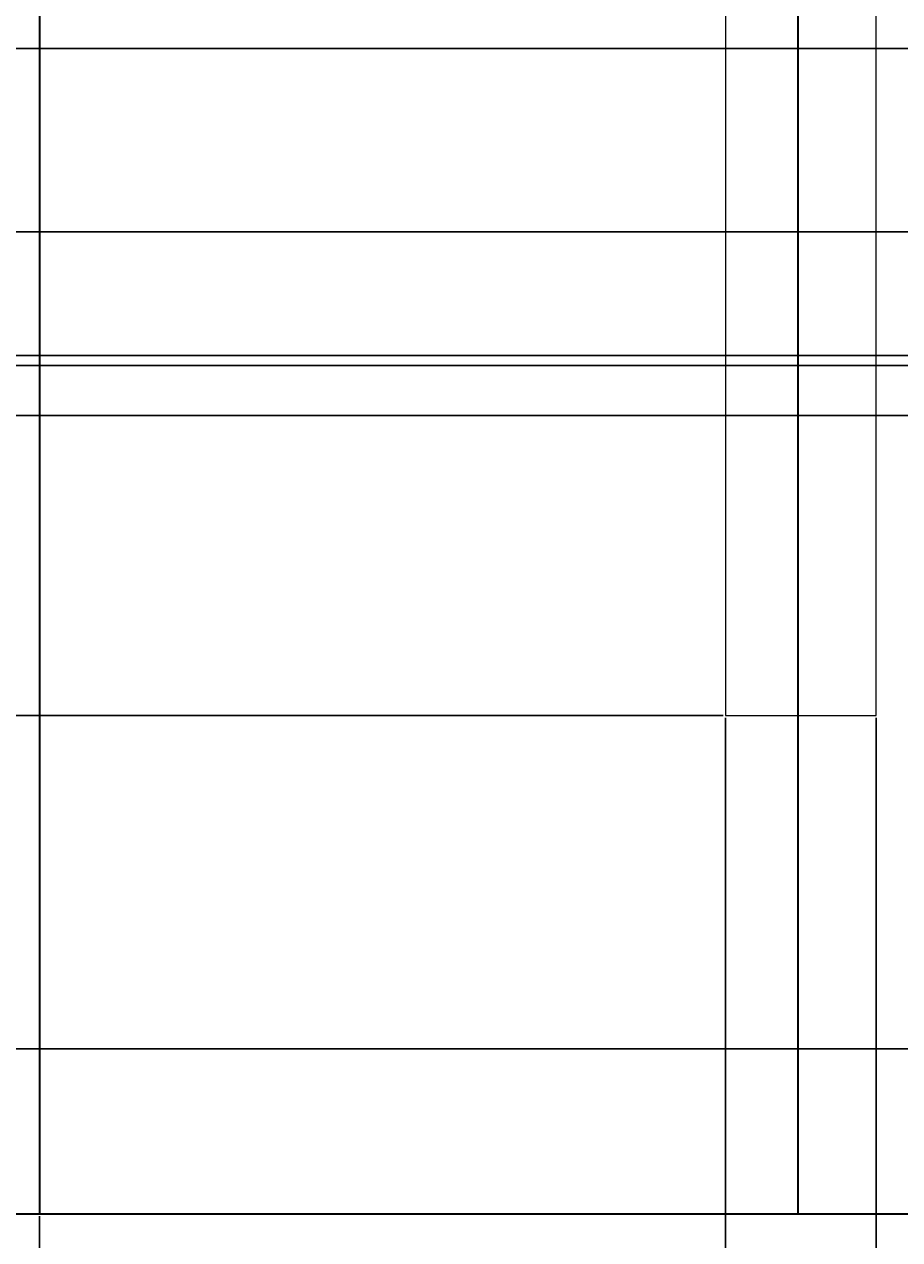
# Model space of a CAD drawing. Units: inches. Extents: x 27 to 200, y -50 to 102.
# Tile 3 of 26: x 44 to 67, y -17 to 15. Entities that reach past the tile are written whole.
import ezdxf

# ---------------------------------------------------------------- set-up
doc = ezdxf.new("R2010")
doc.units = ezdxf.units.IN
doc.header["$MEASUREMENT"] = 0
for name, color, linetype, lineweight in [('A-ANNO-DIMS', 2, 'Continuous', 18), ('A-ELEV', 7, 'Continuous', 35), ('A-EQPM', 9, 'Continuous', 18)]:
    doc.layers.add(name, color=color, linetype=linetype, lineweight=lineweight)
doc.styles.get("Standard").update_dxf_attribs({"font": 'arial.ttf'})
doc.dimstyles.get("Standard").update_dxf_attribs({"dimtxt": 0.18, "dimasz": 0.18, "dimexe": 0.18, "dimexo": 0.0625, "dimgap": 0.09, "dimtad": 0, "dimtih": 1, "dimtoh": 1, "dimdec": 4, "dimzin": 0, "dimdsep": 46, "dimtxsty": 'Standard', "dimcen": 0.09, "dimadec": 0, "dimazin": 0, "dimtfac": 1, "dimtdec": 4, "dimtofl": 0, "dimtmove": 0, "dimatfit": 3, "dimfxl": 1, "dimtolj": 1, "dimtzin": 0, "dimarcsym": 0})

# ---------------------------------------------------------------- blocks, each defined once
blk = doc.blocks.new('*D23')
at = {"layer": 'A-ANNO-DIMS', "color": 0, "lineweight": -2, "transparency": 16777216}
for p, q in [((35.417, -16.832), (35.417, -25.149)), ((191.417, -16.832), (191.417, -25.149)), ((35.597, -24.969), (113.137, -24.969)), ((191.237, -24.969), (113.697, -24.969))]:
    blk.add_line(p, q, dxfattribs=at)
at = {"layer": 'A-ANNO-DIMS', "color": 0, "transparency": 16777216}
for points in [[(35.597, -24.939), (35.597, -24.999), (35.417, -24.969)], [(191.237, -24.939), (191.237, -24.999), (191.417, -24.969)]]:
    blk.add_solid(points, dxfattribs=at)
at = {"layer": 'Defpoints', "color": 0, "transparency": 16777216}
for p in [(35.417, -16.769), (191.417, -16.769), (191.417, -24.969)]:
    blk.add_point(p, dxfattribs=at)
at = {"layer": 'A-ANNO-DIMS', "color": 0, "transparency": 16777216, "insert": (113.417, -24.969), "char_height": 0.18, "attachment_point": 5}
blk.add_mtext('\\A1;156', dxfattribs=at)
blk = doc.blocks.new('*D41')
at = {"layer": 'A-ANNO-DIMS', "color": 0, "lineweight": -2, "transparency": 16777216}
for p, q in [((62.505, -3.679), (62.505, -25.149)), ((44.417, -16.832), (44.417, -25.149)), ((44.597, -24.969), (53.076, -24.969)), ((62.325, -24.969), (53.847, -24.969))]:
    blk.add_line(p, q, dxfattribs=at)
at = {"layer": 'A-ANNO-DIMS', "color": 0, "transparency": 16777216}
for points in [[(44.597, -24.939), (44.597, -24.999), (44.417, -24.969)], [(62.325, -24.939), (62.325, -24.999), (62.505, -24.969)]]:
    blk.add_solid(points, dxfattribs=at)
at = {"layer": 'Defpoints', "color": 0, "transparency": 16777216}
for p in [(62.505, -3.617), (44.417, -16.769), (62.505, -24.969)]:
    blk.add_point(p, dxfattribs=at)
at = {"layer": 'A-ANNO-DIMS', "color": 0, "transparency": 16777216, "insert": (53.461, -24.969), "char_height": 0.18, "attachment_point": 5}
blk.add_mtext('\\A1;18.09', dxfattribs=at)
blk = doc.blocks.new('*D42')
at = {"layer": 'A-ANNO-DIMS', "color": 0, "lineweight": -2, "transparency": 16777216}
for p, q in [((62.505, -3.679), (62.505, -25.149)), ((66.479, -3.679), (66.479, -25.149)), ((62.685, -24.969), (64.098, -24.969)), ((66.299, -24.969), (64.886, -24.969))]:
    blk.add_line(p, q, dxfattribs=at)
at = {"layer": 'A-ANNO-DIMS', "color": 0, "transparency": 16777216}
for points in [[(62.685, -24.939), (62.685, -24.999), (62.505, -24.969)], [(66.299, -24.939), (66.299, -24.999), (66.479, -24.969)]]:
    blk.add_solid(points, dxfattribs=at)
at = {"layer": 'Defpoints', "color": 0, "transparency": 16777216}
for p in [(62.505, -3.617), (66.479, -3.617), (66.479, -24.969)]:
    blk.add_point(p, dxfattribs=at)
at = {"layer": 'A-ANNO-DIMS', "color": 0, "transparency": 16777216, "insert": (64.492, -24.969), "char_height": 0.18, "attachment_point": 5}
blk.add_mtext('\\A1;3.973', dxfattribs=at)
blk = doc.blocks.new('*D43')
at = {"layer": 'A-ANNO-DIMS', "color": 0, "lineweight": -2, "transparency": 16777216}
for p, q in [((66.479, -3.679), (66.479, -25.149)), ((84.417, -16.832), (84.417, -25.149)), ((66.659, -24.969), (75.063, -24.969)), ((84.237, -24.969), (75.833, -24.969))]:
    blk.add_line(p, q, dxfattribs=at)
at = {"layer": 'A-ANNO-DIMS', "color": 0, "transparency": 16777216}
for points in [[(66.659, -24.939), (66.659, -24.999), (66.479, -24.969)], [(84.237, -24.939), (84.237, -24.999), (84.417, -24.969)]]:
    blk.add_solid(points, dxfattribs=at)
at = {"layer": 'Defpoints', "color": 0, "transparency": 16777216}
for p in [(66.479, -3.617), (84.417, -16.769), (84.417, -24.969)]:
    blk.add_point(p, dxfattribs=at)
at = {"layer": 'A-ANNO-DIMS', "color": 0, "transparency": 16777216, "insert": (75.448, -24.969), "char_height": 0.18, "attachment_point": 5}
blk.add_mtext('\\A1;17.94', dxfattribs=at)
blk = doc.blocks.new('*D44')
at = {"layer": 'A-ANNO-DIMS', "color": 0, "lineweight": -2, "transparency": 16777216}
for p, q in [((62.443, -3.617), (27.037, -3.617)), ((27.217, -3.797), (27.217, -10.011)), ((27.217, -16.589), (27.217, -10.375)), ((44.354, -16.769), (27.037, -16.769))]:
    blk.add_line(p, q, dxfattribs=at)
at = {"layer": 'A-ANNO-DIMS', "color": 0, "transparency": 16777216}
for points in [[(27.187, -3.797), (27.247, -3.797), (27.217, -3.617)], [(27.187, -16.589), (27.247, -16.589), (27.217, -16.769)]]:
    blk.add_solid(points, dxfattribs=at)
at = {"layer": 'Defpoints', "color": 0, "transparency": 16777216}
for p in [(27.217, -3.617), (62.505, -3.617), (44.417, -16.769)]:
    blk.add_point(p, dxfattribs=at)
at = {"layer": 'A-ANNO-DIMS', "color": 0, "transparency": 16777216, "insert": (27.217, -10.193), "char_height": 0.18, "attachment_point": 5}
blk.add_mtext('\\A1;13.153', dxfattribs=at)
blk = doc.blocks.new('*D45')
at = {"layer": 'A-ANNO-DIMS', "color": 0, "lineweight": -2, "transparency": 16777216}
for p, q in [((62.443, 26.764), (27.037, 26.764)), ((27.217, 26.584), (27.217, 11.755)), ((27.217, -3.437), (27.217, 11.392)), ((62.443, -3.617), (27.037, -3.617))]:
    blk.add_line(p, q, dxfattribs=at)
at = {"layer": 'A-ANNO-DIMS', "color": 0, "transparency": 16777216}
for points in [[(27.187, 26.584), (27.247, 26.584), (27.217, 26.764)], [(27.187, -3.437), (27.247, -3.437), (27.217, -3.617)]]:
    blk.add_solid(points, dxfattribs=at)
at = {"layer": 'Defpoints', "color": 0, "transparency": 16777216}
for p in [(27.217, 26.764), (62.505, 26.764), (62.505, -3.617)]:
    blk.add_point(p, dxfattribs=at)
at = {"layer": 'A-ANNO-DIMS', "color": 0, "transparency": 16777216, "insert": (27.217, 11.573), "char_height": 0.18, "attachment_point": 5}
blk.add_mtext('\\A1;30.38', dxfattribs=at)
blk = doc.blocks.new('*D54')
at = {"layer": 'A-ANNO-DIMS', "color": 0, "lineweight": -2, "transparency": 16777216}
for p, q in [((120.833, 13.977), (27.037, 13.977)), ((27.217, 13.797), (27.217, 11.743)), ((27.217, 9.324), (27.217, 11.379)), ((120.833, 9.144), (27.037, 9.144))]:
    blk.add_line(p, q, dxfattribs=at)
at = {"layer": 'A-ANNO-DIMS', "color": 0, "transparency": 16777216}
for points in [[(27.187, 13.797), (27.247, 13.797), (27.217, 13.977)], [(27.187, 9.324), (27.247, 9.324), (27.217, 9.144)]]:
    blk.add_solid(points, dxfattribs=at)
at = {"layer": 'Defpoints', "color": 0, "transparency": 16777216}
for p in [(27.217, 13.977), (120.895, 13.977), (120.895, 9.144)]:
    blk.add_point(p, dxfattribs=at)
at = {"layer": 'A-ANNO-DIMS', "color": 0, "transparency": 16777216, "insert": (27.217, 11.561), "char_height": 0.18, "attachment_point": 5}
blk.add_mtext('\\A1;4.83', dxfattribs=at)
blk = doc.blocks.new('*D56')
at = {"layer": 'A-ANNO-DIMS', "color": 0, "lineweight": -2, "transparency": 16777216}
for p, q in [((121.225, 5.878), (27.037, 5.878)), ((27.217, 5.698), (27.217, -3.085)), ((27.217, -12.231), (27.217, -3.448)), ((121.225, -12.411), (27.037, -12.411))]:
    blk.add_line(p, q, dxfattribs=at)
at = {"layer": 'A-ANNO-DIMS', "color": 0, "transparency": 16777216}
for points in [[(27.187, 5.698), (27.247, 5.698), (27.217, 5.878)], [(27.187, -12.231), (27.247, -12.231), (27.217, -12.411)]]:
    blk.add_solid(points, dxfattribs=at)
at = {"layer": 'Defpoints', "color": 0, "transparency": 16777216}
for p in [(27.217, 5.878), (121.288, 5.878), (121.288, -12.411)]:
    blk.add_point(p, dxfattribs=at)
at = {"layer": 'A-ANNO-DIMS', "color": 0, "transparency": 16777216, "insert": (27.217, -3.267), "char_height": 0.18, "attachment_point": 5}
blk.add_mtext('\\A1;18.29', dxfattribs=at)
blk = doc.blocks.new('*D68')
at = {"layer": 'A-ANNO-DIMS', "color": 0, "lineweight": -2, "transparency": 16777216}
for p, q in [((145.153, 5.617), (27.037, 5.617)), ((27.217, 5.437), (27.217, 5.138)), ((27.217, 4.476), (27.217, 4.774)), ((145.153, 4.296), (27.037, 4.296))]:
    blk.add_line(p, q, dxfattribs=at)
at = {"layer": 'A-ANNO-DIMS', "color": 0, "transparency": 16777216}
for points in [[(27.187, 5.437), (27.247, 5.437), (27.217, 5.617)], [(27.187, 4.476), (27.247, 4.476), (27.217, 4.296)]]:
    blk.add_solid(points, dxfattribs=at)
at = {"layer": 'Defpoints', "color": 0, "transparency": 16777216}
for p in [(27.217, 5.617), (145.216, 5.617), (145.216, 4.296)]:
    blk.add_point(p, dxfattribs=at)
at = {"layer": 'A-ANNO-DIMS', "color": 0, "transparency": 16777216, "insert": (27.217, 4.956), "char_height": 0.18, "attachment_point": 5}
blk.add_mtext('\\A1;1.32', dxfattribs=at)
blk = doc.blocks.new('*D69')
at = {"layer": 'A-ANNO-DIMS', "color": 0, "lineweight": -2, "transparency": 16777216}
for p, q in [((121.225, -12.411), (27.037, -12.411)), ((27.217, -12.591), (27.217, -14.408)), ((27.217, -16.589), (27.217, -14.772)), ((119.249, -16.769), (27.037, -16.769))]:
    blk.add_line(p, q, dxfattribs=at)
at = {"layer": 'A-ANNO-DIMS', "color": 0, "transparency": 16777216}
for points in [[(27.187, -12.591), (27.247, -12.591), (27.217, -12.411)], [(27.187, -16.589), (27.247, -16.589), (27.217, -16.769)]]:
    blk.add_solid(points, dxfattribs=at)
at = {"layer": 'Defpoints', "color": 0, "transparency": 16777216}
for p in [(27.217, -12.411), (121.288, -12.411), (119.312, -16.769)]:
    blk.add_point(p, dxfattribs=at)
at = {"layer": 'A-ANNO-DIMS', "color": 0, "transparency": 16777216, "insert": (27.217, -14.59), "char_height": 0.18, "attachment_point": 5}
blk.add_mtext('\\A1;4.358', dxfattribs=at)

msp = doc.modelspace()

# ---------------------------------------------------------------- linework, layer by layer
at = {"layer": 'A-ELEV'}
for p, q in [((44.4169, 44.9264), (44.4169, -16.7693)), ((64.4169, 44.9264), (64.4169, -16.7693)), ((35.4169, -16.7693), (191.4169, -16.7693))]:
    msp.add_line(p, q, dxfattribs=at)
at = {"layer": 'A-EQPM'}
for points in [[(64.4169, 26.7638), (62.5054, 26.7638), (62.5054, -3.6168), (64.4169, -3.6168)], [(64.4169, -3.6168), (66.4786, -3.6168), (66.4786, 26.7638), (64.4169, 26.7638)]]:
    msp.add_lwpolyline(points, close=True, dxfattribs=at)

# ---------------------------------------------------------------- dimensions: what is measured, and where the dimension line sits
at = {"layer": 'A-ANNO-DIMS'}
for base, p1, p2, override, picture, middle in [((27.2169, 26.7638), (62.5054, -3.6168), (62.5054, 26.7638), {"dimdec": 2, "dimlfac": 1, "dimrnd": 0, "dimzin": 0, "dimdsep": 46, "dimlunit": 2}, '*D45', (27.2169, 11.5735)), ((27.2169, 13.9773), (120.8954, 9.1438), (120.8954, 13.9773), {"dimdec": 2, "dimlfac": 1, "dimrnd": 0, "dimzin": 0, "dimdsep": 46, "dimlunit": 2}, '*D54', (27.2169, 11.5606)), ((27.2169, 5.8779), (121.2876, -12.411), (121.2876, 5.8779), {"dimdec": 2, "dimlfac": 1, "dimrnd": 0, "dimzin": 0, "dimdsep": 46, "dimlunit": 2}, '*D56', (27.2169, -3.2665)), ((27.2169, 5.6167), (145.216, 4.2959), (145.216, 5.6167), {"dimdec": 2, "dimlfac": 1, "dimrnd": 0, "dimzin": 0, "dimdsep": 46, "dimlunit": 2}, '*D68', (27.2169, 4.9563)), ((27.216902, -3.61681), (44.416902, -16.76931), (62.505395, -3.61681), {"dimdec": 3, "dimlfac": 1, "dimrnd": 0, "dimzin": 0, "dimdsep": 46, "dimlunit": 2}, '*D44', (27.216902, -10.19306)), ((27.2169, -12.411), (119.3118, -16.7693), (121.2876, -12.411), {"dimdec": 3, "dimlfac": 1, "dimrnd": 0, "dimzin": 0, "dimdsep": 46, "dimlunit": 2}, '*D69', (27.2169, -14.5901))]:
    dim = msp.add_linear_dim(base=base, p1=p1, p2=p2, angle=90, dimstyle='Standard', override=override, dxfattribs=at)
    dim.commit()
    dim.dimension.update_dxf_attribs({"geometry": picture, "text_midpoint": middle})
for base, p1, p2, override, picture, middle in [((62.5054, -24.9693), (44.4169, -16.7693), (62.5054, -3.6168), {"dimdec": 2, "dimlfac": 1, "dimrnd": 0, "dimzin": 0, "dimdsep": 46, "dimlunit": 2}, '*D41', (53.4611, -24.9693)), ((66.4786, -24.9693), (62.5054, -3.6168), (66.4786, -3.6168), {"dimdec": 3, "dimlfac": 1, "dimrnd": 0, "dimzin": 0, "dimdsep": 46, "dimlunit": 2}, '*D42', (64.492, -24.9693)), ((84.4169, -24.9693), (66.4786, -3.6168), (84.4169, -16.7693), {"dimdec": 2, "dimlfac": 1, "dimrnd": 0, "dimzin": 0, "dimdsep": 46, "dimlunit": 2}, '*D43', (75.4478, -24.9693)), ((191.4169, -24.9693), (35.4169, -16.7693), (191.4169, -16.7693), {"dimdec": 0, "dimlfac": 1, "dimrnd": 0, "dimzin": 0, "dimdsep": 46, "dimlunit": 2}, '*D23', (113.4169, -24.9693))]:
    dim = msp.add_linear_dim(base=base, p1=p1, p2=p2, dimstyle='Standard', override=override, dxfattribs=at)
    dim.commit()
    dim.dimension.update_dxf_attribs({"geometry": picture, "text_midpoint": middle})

doc.saveas('drawing.dxf')
